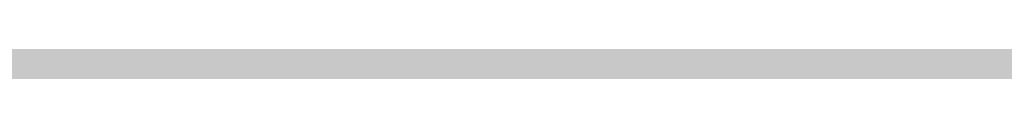
# Model space of a CAD drawing. Units: millimetres. Extents: x 0 to 2267, y 0 to 1823.
# Tile 198 of 256: x 1838.83 to 1841.442, y 1127.423 to 1127.462. Entities that reach past the tile are written whole.
import ezdxf

# ---------------------------------------------------------------- set-up
doc = ezdxf.new("R2010")
doc.units = ezdxf.units.MM
doc.header["$MEASUREMENT"] = 0
doc.layers.add('M-HATC', color=252, linetype='Continuous', lineweight=18)

msp = doc.modelspace()

# ---------------------------------------------------------------- hatches: boundary and pattern name
at = {"layer": 'M-HATC'}
h = msp.add_hatch(color=256, dxfattribs=at)
h.dxf.hatch_style = 1
h.paths.add_polyline_path([(2055.771, 1603.062), (1381.0868, 1603.062), (1381.0868, 1598.062), (2055.771, 1598.062)])
h.paths.add_polyline_path([(2055.771, 1598.062), (1381.0868, 1598.062), (1381.0868, 1593.062), (2055.771, 1593.062)])
h.paths.add_polyline_path([(2051.3074, 1536.7609), (1385.5504, 1536.7609), (1385.5504, 1526.7609), (1387.5504, 1526.7609), (1388.5366, 1525.0528), (1385.3319, 1521.2335), (1385.3319, 1521.2226), (2050.2542, 1522.7491), (2048.3212, 1525.0528), (2049.3074, 1526.7609), (2051.3074, 1526.7609)])
edge = h.paths.add_edge_path()
edge.add_arc((1847.5345, 1379.1492), 135, 222.603061, 222.890851, ccw=False)
edge.add_line((1748.1663, 1287.7656), (1683.0921, 1287.7656))
edge.add_arc((1583.7239, 1379.1492), 135, 317.109149, 317.396939, ccw=False)
edge.add_arc((1678.9686, 1290.6707), 5, 222.8909, 317.1091, ccw=False)
edge.add_arc((1774.2133, 1379.1492), 135, 222.603061, 222.890851, ccw=False)
edge.add_line((1674.8451, 1287.7656), (1609.7709, 1287.7656))
edge.add_arc((1510.4027, 1379.1492), 135, 317.109149, 317.396939, ccw=False)
edge.add_arc((1605.6474, 1290.6707), 5, 222.8909, 317.1091, ccw=False)
edge.add_arc((1700.8921, 1379.1492), 135, 222.603061, 222.890851, ccw=False)
edge.add_line((1601.5239, 1287.7656), (1536.4497, 1287.7656))
edge.add_arc((1437.0815, 1379.1492), 135, 317.109149, 317.396939, ccw=False)
edge.add_arc((1532.3262, 1290.6707), 5, 222.8909, 317.1091, ccw=False)
edge.add_arc((1627.5709, 1379.1492), 135, 222.603061, 222.890851, ccw=False)
edge.add_line((1528.2027, 1287.7656), (1505.9289, 1287.7656))
edge.add_spline(control_points=[(1505.9289, 1287.7656), (1504.2622, 1287.7656), (1504.2622, 1282.7656), (1505.9289, 1282.7656)], knot_values=[0, 0, 0, 0, 5, 5, 5, 5], degree=3, periodic=0)
edge.add_line((1505.9289, 1282.7656), (1930.9289, 1282.7656))
edge.add_spline(control_points=[(1930.9289, 1282.7656), (1932.5956, 1282.7656), (1932.5956, 1287.7656), (1930.9289, 1287.7656)], knot_values=[0, 0, 0, 0, 5, 5, 5, 5], degree=3, periodic=0)
edge.add_line((1930.9289, 1287.7656), (1903.0557, 1287.7656))
edge.add_arc((1803.6875, 1379.1492), 135, 317.109149, 317.396939, ccw=False)
edge.add_arc((1898.9322, 1290.6707), 5, 222.8909, 317.1091, ccw=False)
edge.add_arc((1994.1769, 1379.1492), 135, 222.603061, 222.890851, ccw=False)
edge.add_line((1894.8087, 1287.7656), (1829.7345, 1287.7656))
edge.add_arc((1730.3663, 1379.1492), 135, 317.109149, 317.396939, ccw=False)
edge.add_arc((1825.611, 1290.6707), 5, 222.8909, 317.1091, ccw=False)
edge.add_arc((1920.8557, 1379.1492), 135, 222.603061, 222.890851, ccw=False)
edge.add_line((1821.4875, 1287.7656), (1756.4133, 1287.7656))
edge.add_arc((1657.0451, 1379.1492), 135, 317.109149, 317.396939, ccw=False)
edge.add_arc((1752.2898, 1290.6707), 5, 222.8909, 317.1091, ccw=False)
edge = h.paths.add_edge_path()
edge.add_spline(control_points=[(1843.4289, 1227.2475), (1845.0956, 1227.2475), (1845.0956, 1232.2475), (1843.4289, 1232.2475)], knot_values=[0, 0, 0, 0, 5, 5, 5, 5], degree=3, periodic=0)
edge.add_line((1843.4289, 1232.2475), (1593.4289, 1232.2475))
edge.add_spline(control_points=[(1593.4289, 1232.2475), (1591.7622, 1232.2475), (1591.7622, 1227.2475), (1593.4289, 1227.2475)], knot_values=[0, 0, 0, 0, 5, 5, 5, 5], degree=3, periodic=0)
edge.add_line((1593.4289, 1227.2475), (1843.4289, 1227.2475))
h.paths.add_polyline_path([(1905.9289, 1127.4171), (1530.9289, 1127.4171, 0.414214), (1520.9289, 1117.4171), (1530.9289, 1117.4171), (1915.9289, 1117.4171, 0.414214)])
edge = h.paths.add_edge_path()
edge.add_arc((1397.0858, 1498.4078), 12.7299, 90.78215, 190.87871, ccw=False)
edge.add_line((1396.912, 1511.1365), (1428.0097, 1511.3488))
edge.add_line((1428.0097, 1511.3488), (1433.0097, 1511.3488))
edge.add_line((1433.0097, 1511.3488), (1434.439, 1511.3488))
edge.add_arc((1419.474, 1498.0804), 20, 41.561, 74.08211)
edge.add_line((1424.9592, 1517.3135), (1399.9351, 1517.2561))
edge.add_spline(control_points=[(1399.9307, 1517.2561), (1399.884, 1517.2131), (1399.8328, 1517.1689), (1399.7774, 1517.1236)], knot_values=[11.567499, 11.567499, 11.567499, 11.567499, 11.814249, 11.814249, 11.814249, 11.814249], degree=3, periodic=0)
edge.add_spline(control_points=[(1399.6328, 1517.0099), (1399.5831, 1516.9721), (1399.5307, 1516.9338), (1399.4759, 1516.8947)], knot_values=[11.167718, 11.167718, 11.167718, 11.167718, 11.365188, 11.365188, 11.365188, 11.365188], degree=3, periodic=0)
edge.add_spline(control_points=[(1399.3398, 1516.8001), (1399.1514, 1516.6719), (1398.9384, 1516.5377), (1398.704, 1516.3994)], knot_values=[10.376405, 10.376405, 10.376405, 10.376405, 11.00994, 11.00994, 11.00994, 11.00994], degree=3, periodic=0)
edge.add_spline(control_points=[(1398.6572, 1516.3719), (1398.5789, 1516.326), (1398.4983, 1516.2797), (1398.4155, 1516.2331)], knot_values=[10.125175, 10.125175, 10.125175, 10.125175, 10.334406, 10.334406, 10.334406, 10.334406], degree=3, periodic=0)
edge.add_spline(control_points=[(1398.2642, 1516.1487), (1398.196, 1516.1111), (1398.1263, 1516.0732), (1398.0555, 1516.0351)], knot_values=[9.832246, 9.832246, 9.832246, 9.832246, 9.999658, 9.999658, 9.999658, 9.999658], degree=3, periodic=0)
edge.add_spline(control_points=[(1397.9987, 1516.0048), (1397.7312, 1515.8621), (1397.446, 1515.7171), (1397.1466, 1515.5714)], knot_values=[9.161808, 9.161808, 9.161808, 9.161808, 9.787769, 9.787769, 9.787769, 9.787769], degree=3, periodic=0)
edge.add_spline(control_points=[(1397.1466, 1515.5714), (1396.8418, 1515.423), (1396.5222, 1515.274), (1396.1914, 1515.1262)], knot_values=[8.524455, 8.524455, 8.524455, 8.524455, 9.161808, 9.161808, 9.161808, 9.161808], degree=3, periodic=0)
edge.add_spline(control_points=[(1396.0777, 1515.0756), (1395.9854, 1515.0348), (1395.8922, 1514.994), (1395.7983, 1514.9534)], knot_values=[8.275193, 8.275193, 8.275193, 8.275193, 8.451726, 8.451726, 8.451726, 8.451726], degree=3, periodic=0)
edge.add_spline(control_points=[(1395.6018, 1514.8691), (1395.4997, 1514.8257), (1395.3968, 1514.7824), (1395.2932, 1514.7394)], knot_values=[7.962917, 7.962917, 7.962917, 7.962917, 8.152764, 8.152764, 8.152764, 8.152764], degree=3, periodic=0)
edge.add_spline(control_points=[(1395.2116, 1514.7057), (1394.8278, 1514.5475), (1394.4345, 1514.3929), (1394.0364, 1514.2442)], knot_values=[7.21254, 7.21254, 7.21254, 7.21254, 7.913148, 7.913148, 7.913148, 7.913148], degree=3, periodic=0)
edge.add_spline(control_points=[(1394.0364, 1514.2442), (1393.7076, 1514.1214), (1393.3754, 1514.0027), (1393.0427, 1513.8895)], knot_values=[6.633733, 6.633733, 6.633733, 6.633733, 7.21254, 7.21254, 7.21254, 7.21254], degree=3, periodic=0)
edge.add_spline(control_points=[(1392.8214, 1513.815), (1392.7198, 1513.7812), (1392.6181, 1513.7479), (1392.5166, 1513.7152)], knot_values=[6.328796, 6.328796, 6.328796, 6.328796, 6.505493, 6.505493, 6.505493, 6.505493], degree=3, periodic=0)
edge.add_spline(control_points=[(1392.5166, 1513.7152), (1392.3187, 1513.6515), (1392.1212, 1513.59), (1391.9244, 1513.531)], knot_values=[5.984605, 5.984605, 5.984605, 5.984605, 6.328796, 6.328796, 6.328796, 6.328796], degree=3, periodic=0)
edge.add_spline(control_points=[(1391.7915, 1513.4915), (1391.3122, 1513.3501), (1390.8384, 1513.2239), (1390.3784, 1513.1171)], knot_values=[5.066697, 5.066697, 5.066697, 5.066697, 5.907055, 5.907055, 5.907055, 5.907055], degree=3, periodic=0)
edge.add_spline(control_points=[(1390.3784, 1513.1171), (1390.1797, 1513.071), (1389.9836, 1513.0284), (1389.7907, 1512.9899)], knot_values=[4.70367, 4.70367, 4.70367, 4.70367, 5.066695, 5.066695, 5.066695, 5.066695], degree=3, periodic=0)
edge.add_spline(control_points=[(1389.422, 1512.9204), (1389.2459, 1512.8892), (1389.0729, 1512.8617), (1388.9036, 1512.8381)], knot_values=[4.130571, 4.130571, 4.130571, 4.130571, 4.469816, 4.469816, 4.469816, 4.469816], degree=3, periodic=0)
edge.add_spline(control_points=[(1388.9036, 1512.8381), (1388.591, 1512.7946), (1388.2911, 1512.7644), (1388.0071, 1512.7494)], knot_values=[3.504031, 3.504031, 3.504031, 3.504031, 4.130571, 4.130571, 4.130571, 4.130571], degree=3, periodic=0)
edge.add_spline(control_points=[(1387.9356, 1512.7459), (1387.8538, 1512.7423), (1387.7733, 1512.74), (1387.6944, 1512.739)], knot_values=[3.268866, 3.268866, 3.268866, 3.268866, 3.451164, 3.451164, 3.451164, 3.451164], degree=3, periodic=0)
edge.add_spline(control_points=[(1387.3351, 1512.7443), (1387.2076, 1512.7499), (1387.0847, 1512.7597), (1386.967, 1512.7739)], knot_values=[2.670686, 2.670686, 2.670686, 2.670686, 2.984, 2.984, 2.984, 2.984], degree=3, periodic=0)
edge.add_spline(control_points=[(1386.8327, 1512.7922), (1386.8209, 1512.7941), (1386.8092, 1512.7959), (1386.7975, 1512.7979)], knot_values=[2.516981, 2.516981, 2.516981, 2.516981, 2.549528, 2.549528, 2.549528, 2.549528], degree=3, periodic=0)
edge.add_spline(control_points=[(1386.4526, 1512.8735), (1386.4257, 1512.881), (1386.3993, 1512.889), (1386.3733, 1512.8972)], knot_values=[2.095869, 2.095869, 2.095869, 2.095869, 2.17941, 2.17941, 2.17941, 2.17941], degree=3, periodic=0)
edge.add_spline(control_points=[(1386.0691, 1513.0189), (1386.0634, 1513.0217), (1386.0577, 1513.0246), (1386.052, 1513.0275)], knot_values=[1.72453, 1.72453, 1.72453, 1.72453, 1.745933, 1.745933, 1.745933, 1.745933], degree=3, periodic=0)
edge.add_arc((1399.474, 1498.0804), 20, 131.82432, 180)
edge.add_arc((1630.3336, 1505.5484), 250.9708, 181.705176, 236.427975)
edge.add_arc((1605.3399, 1483.3044), 218.7822, 238.660829, 243.34961)
edge.add_arc((1647.0911, 1510.3592), 262.8986, 183.129836, 237.853442, ccw=False)
h.paths.add_polyline_path([(1406.5369, 1391.9644, 0.149382), (1491.5506, 1296.4418, -0.129517)], flags=17)
edge = h.paths.add_edge_path()
edge.add_arc((2037.3838, 1498.0804), 20, 0, 48.26587)
edge.add_spline(control_points=[(2050.6973, 1513.0052), (2050.6512, 1512.9847), (2050.6034, 1512.9655), (2050.5539, 1512.9477)], knot_values=[1.835652, 1.835652, 1.835652, 1.835652, 2.000781, 2.000781, 2.000781, 2.000781], degree=3, periodic=0)
edge.add_spline(control_points=[(2050.4616, 1512.9166), (2050.479, 1512.9221), (2050.4963, 1512.9277), (2050.5133, 1512.9335)], knot_values=[2.045477, 2.045477, 2.045477, 2.045477, 2.101389, 2.101389, 2.101389, 2.101389], degree=3, periodic=0)
edge.add_spline(control_points=[(2050.129, 1512.8342), (2050.1984, 1512.8473), (2050.2657, 1512.8623), (2050.3308, 1512.8792)], knot_values=[2.237629, 2.237629, 2.237629, 2.237629, 2.435841, 2.435841, 2.435841, 2.435841], degree=3, periodic=0)
edge.add_spline(control_points=[(2050.0946, 1512.8278), (2050.1061, 1512.8299), (2050.1176, 1512.832), (2050.129, 1512.8342)], knot_values=[2.435841, 2.435841, 2.435841, 2.435841, 2.468321, 2.468321, 2.468321, 2.468321], degree=3, periodic=0)
edge.add_spline(control_points=[(2049.7843, 1512.7851), (2049.8552, 1512.7922), (2049.9243, 1512.8008), (2049.9917, 1512.8109)], knot_values=[2.563852, 2.563852, 2.563852, 2.563852, 2.748541, 2.748541, 2.748541, 2.748541], degree=3, periodic=0)
edge.add_spline(control_points=[(2049.4052, 1512.7617), (2049.5364, 1512.7653), (2049.6629, 1512.773), (2049.7843, 1512.7851)], knot_values=[2.748541, 2.748541, 2.748541, 2.748541, 3.064882, 3.064882, 3.064882, 3.064882], degree=3, periodic=0)
edge.add_spline(control_points=[(2049.1698, 1512.7597), (2049.2336, 1512.7591), (2049.2965, 1512.7594), (2049.3584, 1512.7606)], knot_values=[3.102309, 3.102309, 3.102309, 3.102309, 3.2503, 3.2503, 3.2503, 3.2503], degree=3, periodic=0)
edge.add_spline(control_points=[(2048.8573, 1512.7691), (2048.9638, 1512.7638), (2049.068, 1512.7606), (2049.1698, 1512.7597)], knot_values=[3.2503, 3.2503, 3.2503, 3.2503, 3.486069, 3.486069, 3.486069, 3.486069], degree=3, periodic=0)
edge.add_spline(control_points=[(2048.6924, 1512.7789), (2048.3729, 1512.8009), (2048.0345, 1512.8411), (2047.6817, 1512.897)], knot_values=[3.606429, 3.606429, 3.606429, 3.606429, 4.2989, 4.2989, 4.2989, 4.2989], degree=3, periodic=0)
edge.add_spline(control_points=[(2047.6817, 1512.897), (2047.5458, 1512.9185), (2047.4077, 1512.9424), (2047.2678, 1512.9685)], knot_values=[4.2989, 4.2989, 4.2989, 4.2989, 4.565769, 4.565769, 4.565769, 4.565769], degree=3, periodic=0)
edge.add_spline(control_points=[(2047.2678, 1512.9685), (2047.1449, 1512.9914), (2047.0207, 1513.016), (2046.8951, 1513.0422)], knot_values=[4.565769, 4.565769, 4.565769, 4.565769, 4.799971, 4.799971, 4.799971, 4.799971], degree=3, periodic=0)
edge.add_spline(control_points=[(2046.8951, 1513.0422), (2046.5286, 1513.1188), (2046.1513, 1513.209), (2045.7676, 1513.3107)], knot_values=[4.799971, 4.799971, 4.799971, 4.799971, 5.483718, 5.483718, 5.483718, 5.483718], degree=3, periodic=0)
edge.add_spline(control_points=[(2045.7676, 1513.3107), (2045.3724, 1513.4154), (2044.9704, 1513.5322), (2044.5662, 1513.6588)], knot_values=[5.483718, 5.483718, 5.483718, 5.483718, 6.187866, 6.187866, 6.187866, 6.187866], degree=3, periodic=0)
edge.add_spline(control_points=[(2044.5662, 1513.6588), (2044.4149, 1513.7061), (2044.2633, 1513.7549), (2044.1116, 1513.8048)], knot_values=[6.187866, 6.187866, 6.187866, 6.187866, 6.451551, 6.451551, 6.451551, 6.451551], degree=3, periodic=0)
edge.add_spline(control_points=[(2044.1116, 1513.8048), (2043.9967, 1513.8427), (2043.8817, 1513.8813), (2043.7668, 1513.9205)], knot_values=[6.451551, 6.451551, 6.451551, 6.451551, 6.651434, 6.651434, 6.651434, 6.651434], degree=3, periodic=0)
edge.add_spline(control_points=[(2043.7668, 1513.9205), (2043.3716, 1514.0554), (2042.9774, 1514.1979), (2042.5886, 1514.3458)], knot_values=[6.651434, 6.651434, 6.651434, 6.651434, 7.338879, 7.338879, 7.338879, 7.338879], degree=3, periodic=0)
edge.add_spline(control_points=[(2042.5886, 1514.3458), (2042.1643, 1514.5071), (2041.7465, 1514.6749), (2041.3409, 1514.846)], knot_values=[7.338879, 7.338879, 7.338879, 7.338879, 8.089209, 8.089209, 8.089209, 8.089209], degree=3, periodic=0)
edge.add_spline(control_points=[(2041.3409, 1514.846), (2041.1028, 1514.9465), (2040.869, 1515.0481), (2040.6405, 1515.1502)], knot_values=[8.089209, 8.089209, 8.089209, 8.089209, 8.529587, 8.529587, 8.529587, 8.529587], degree=3, periodic=0)
edge.add_spline(control_points=[(2040.51, 1515.2089), (2040.0824, 1515.4022), (2039.6747, 1515.5971), (2039.295, 1515.7894)], knot_values=[8.613818, 8.613818, 8.613818, 8.613818, 9.44571, 9.44571, 9.44571, 9.44571], degree=3, periodic=0)
edge.add_spline(control_points=[(2039.295, 1515.7894), (2039.0618, 1515.9075), (2038.8391, 1516.0246), (2038.6288, 1516.1398)], knot_values=[9.44571, 9.44571, 9.44571, 9.44571, 9.956404, 9.956404, 9.956404, 9.956404], degree=3, periodic=0)
edge.add_spline(control_points=[(2038.6288, 1516.1398), (2038.5187, 1516.2001), (2038.4121, 1516.2598), (2038.309, 1516.3189)], knot_values=[9.956404, 9.956404, 9.956404, 9.956404, 10.223542, 10.223542, 10.223542, 10.223542], degree=3, periodic=0)
edge.add_spline(control_points=[(2038.309, 1516.3189), (2038.2138, 1516.3735), (2038.1216, 1516.4276), (2038.0328, 1516.481)], knot_values=[10.223542, 10.223542, 10.223542, 10.223542, 10.47051, 10.47051, 10.47051, 10.47051], degree=3, periodic=0)
edge.add_spline(control_points=[(2038.0328, 1516.481), (2037.7855, 1516.6296), (2037.5639, 1516.773), (2037.3722, 1516.909)], knot_values=[10.47051, 10.47051, 10.47051, 10.47051, 11.15767, 11.15767, 11.15767, 11.15767], degree=3, periodic=0)
edge.add_spline(control_points=[(2037.3722, 1516.909), (2037.2789, 1516.9752), (2037.1927, 1517.0396), (2037.1142, 1517.102)], knot_values=[11.15767, 11.15767, 11.15767, 11.15767, 11.49227, 11.49227, 11.49227, 11.49227], degree=3, periodic=0)
edge.add_spline(control_points=[(2036.8564, 1517.3259), (2036.9148, 1517.2692), (2036.9814, 1517.2103), (2037.0557, 1517.1492)], knot_values=[11.577341, 11.577341, 11.577341, 11.577341, 11.91035, 11.91035, 11.91035, 11.91035], degree=3, periodic=0)
edge.add_spline(control_points=[(2036.8074, 1517.3748), (2036.823, 1517.3587), (2036.8393, 1517.3424), (2036.8564, 1517.3259)], knot_values=[11.91035, 11.91035, 11.91035, 11.91035, 12.007402, 12.007402, 12.007402, 12.007402], degree=3, periodic=0)
edge.add_spline(control_points=[(2036.7017, 1517.494), (2036.7104, 1517.483), (2036.7196, 1517.4719), (2036.7291, 1517.4606)], knot_values=[12.184155, 12.184155, 12.184155, 12.184155, 12.255409, 12.255409, 12.255409, 12.255409], degree=3, periodic=0)
edge.add_spline(control_points=[(2036.6159, 1517.6205), (2036.62, 1517.613), (2036.6243, 1517.6055), (2036.6289, 1517.5979)], knot_values=[12.487913, 12.487913, 12.487913, 12.487913, 12.541035, 12.541035, 12.541035, 12.541035], degree=3, periodic=0)
edge.add_spline(control_points=[(2036.5635, 1517.786), (2036.5637, 1517.7794), (2036.5642, 1517.7726), (2036.565, 1517.7658)], knot_values=[12.911761, 12.911761, 12.911761, 12.911761, 12.968286, 12.968286, 12.968286, 12.968286], degree=3, periodic=0)
edge.add_spline(control_points=[(2036.6166, 1517.9304), (2036.6125, 1517.9259), (2036.6086, 1517.9212), (2036.6049, 1517.9165)], knot_values=[13.382527, 13.382527, 13.382527, 13.382527, 13.433791, 13.433791, 13.433791, 13.433791], degree=3, periodic=0)
edge.add_spline(control_points=[(2036.749, 1518.017), (2036.7361, 1518.0116), (2036.7239, 1518.006), (2036.7124, 1518.0002)], knot_values=[13.726299, 13.726299, 13.726299, 13.726299, 13.809928, 13.809928, 13.809928, 13.809928], degree=3, periodic=0)
edge.add_spline(control_points=[(2036.8604, 1518.0528), (2036.8386, 1518.0474), (2036.8181, 1518.0416), (2036.7988, 1518.0353)], knot_values=[13.910887, 13.910887, 13.910887, 13.910887, 14.02153, 14.02153, 14.02153, 14.02153], degree=3, periodic=0)
edge.add_line((2036.9639, 1518.0804), (2032.3838, 1518.0804))
edge.add_line((2032.3838, 1518.0804), (2027.3838, 1518.0804))
edge.add_line((2027.3838, 1518.0804), (2022.3838, 1518.0804))
edge.add_line((2022.3838, 1518.0804), (2017.3838, 1518.0804))
edge.add_arc((2017.3838, 1498.0804), 20, 90, 138.439)
edge.add_line((2002.4188, 1511.3488), (2003.8481, 1511.3488))
edge.add_line((2003.8481, 1511.3488), (2008.8481, 1511.3488))
edge.add_line((2008.8481, 1511.3488), (2039.772, 1511.1377))
edge.add_arc((2039.772, 1498.4078), 12.7299, -10.87871, 90, ccw=False)
edge.add_arc((1789.7668, 1510.3592), 262.8986, 302.146558, 356.870164, ccw=False)
edge.add_arc((1831.5179, 1483.3044), 218.7822, 296.65039, 301.339171)
edge.add_arc((1806.5242, 1505.5484), 250.9708, 303.572025, 358.294824)
h.paths.add_polyline_path([(2030.321, 1391.9644, -0.129517), (1945.3072, 1296.4418, 0.149382)], flags=17)
edge = h.paths.add_edge_path()
edge.add_spline(control_points=[(2037.2464, 1518.0821), (2037.2898, 1518.081), (2037.3355, 1518.0804), (2037.3838, 1518.0804)], knot_values=[0.000012, 0.000012, 0.000012, 0.000012, 0.144754, 0.144754, 0.144754, 0.144754], degree=3, periodic=0)
edge.add_line((2037.3357, 1518.0804), (2037.0096, 1518.0804))
edge.add_spline(control_points=[(2037.0096, 1518.0804), (2036.9822, 1518.0768), (2036.956, 1518.0727), (2036.9312, 1518.0681)], knot_values=[14.13465, 14.13465, 14.13465, 14.13465, 14.247197, 14.247197, 14.247197, 14.247197], degree=3, periodic=0)
edge.add_spline(control_points=[(2036.9312, 1518.0681), (2036.9276, 1518.0674), (2036.9241, 1518.0667), (2036.9205, 1518.0661)], knot_values=[14.118315, 14.118315, 14.118315, 14.118315, 14.13465, 14.13465, 14.13465, 14.13465], degree=3, periodic=0)
edge.add_spline(control_points=[(2036.9205, 1518.0661), (2036.9118, 1518.0644), (2036.9032, 1518.0626), (2036.8948, 1518.0608)], knot_values=[14.078086, 14.078086, 14.078086, 14.078086, 14.118315, 14.118315, 14.118315, 14.118315], degree=3, periodic=0)
edge.add_spline(control_points=[(2036.8948, 1518.0608), (2036.883, 1518.0583), (2036.8716, 1518.0556), (2036.8604, 1518.0528)], knot_values=[14.02153, 14.02153, 14.02153, 14.02153, 14.078086, 14.078086, 14.078086, 14.078086], degree=3, periodic=0)
edge.add_spline(control_points=[(2036.8604, 1518.0528), (2036.8386, 1518.0474), (2036.8181, 1518.0416), (2036.7988, 1518.0353)], knot_values=[13.910887, 13.910887, 13.910887, 13.910887, 14.02153, 14.02153, 14.02153, 14.02153], degree=3, periodic=0)
edge.add_spline(control_points=[(2036.7988, 1518.0353), (2036.7981, 1518.035), (2036.7974, 1518.0348), (2036.7967, 1518.0346)], knot_values=[13.906906, 13.906906, 13.906906, 13.906906, 13.910887, 13.910887, 13.910887, 13.910887], degree=3, periodic=0)
edge.add_spline(control_points=[(2036.7967, 1518.0346), (2036.7882, 1518.0318), (2036.7799, 1518.0289), (2036.7719, 1518.0259)], knot_values=[13.857826, 13.857826, 13.857826, 13.857826, 13.906906, 13.906906, 13.906906, 13.906906], degree=3, periodic=0)
edge.add_spline(control_points=[(2036.7719, 1518.0259), (2036.764, 1518.023), (2036.7564, 1518.02), (2036.749, 1518.017)], knot_values=[13.809928, 13.809928, 13.809928, 13.809928, 13.857826, 13.857826, 13.857826, 13.857826], degree=3, periodic=0)
edge.add_spline(control_points=[(2036.749, 1518.017), (2036.7361, 1518.0116), (2036.7239, 1518.006), (2036.7124, 1518.0002)], knot_values=[13.726299, 13.726299, 13.726299, 13.726299, 13.809928, 13.809928, 13.809928, 13.809928], degree=3, periodic=0)
edge.add_spline(control_points=[(2036.7124, 1518.0002), (2036.7121, 1518), (2036.7118, 1517.9999), (2036.7115, 1517.9997)], knot_values=[13.723993, 13.723993, 13.723993, 13.723993, 13.726299, 13.726299, 13.726299, 13.726299], degree=3, periodic=0)
edge.add_spline(control_points=[(2036.7115, 1517.9997), (2036.7063, 1517.9971), (2036.7013, 1517.9944), (2036.6965, 1517.9917)], knot_values=[13.686536, 13.686536, 13.686536, 13.686536, 13.723993, 13.723993, 13.723993, 13.723993], degree=3, periodic=0)
edge.add_spline(control_points=[(2036.6965, 1517.9917), (2036.6919, 1517.9891), (2036.6874, 1517.9865), (2036.6831, 1517.9839)], knot_values=[13.651251, 13.651251, 13.651251, 13.651251, 13.686536, 13.686536, 13.686536, 13.686536], degree=3, periodic=0)
edge.add_spline(control_points=[(2036.6831, 1517.9839), (2036.6764, 1517.9798), (2036.67, 1517.9757), (2036.6639, 1517.9714)], knot_values=[13.596804, 13.596804, 13.596804, 13.596804, 13.651251, 13.651251, 13.651251, 13.651251], degree=3, periodic=0)
edge.add_spline(control_points=[(2036.6639, 1517.9714), (2036.6636, 1517.9712), (2036.6633, 1517.9709), (2036.6629, 1517.9707)], knot_values=[13.593956, 13.593956, 13.593956, 13.593956, 13.596804, 13.596804, 13.596804, 13.596804], degree=3, periodic=0)
edge.add_spline(control_points=[(2036.6629, 1517.9707), (2036.6603, 1517.9689), (2036.6577, 1517.967), (2036.6552, 1517.9651)], knot_values=[13.570322, 13.570322, 13.570322, 13.570322, 13.593956, 13.593956, 13.593956, 13.593956], degree=3, periodic=0)
edge.add_spline(control_points=[(2036.6552, 1517.9651), (2036.6525, 1517.9631), (2036.6499, 1517.9611), (2036.6474, 1517.9591)], knot_values=[13.545477, 13.545477, 13.545477, 13.545477, 13.570322, 13.570322, 13.570322, 13.570322], degree=3, periodic=0)
edge.add_spline(control_points=[(2036.6474, 1517.9591), (2036.6472, 1517.9589), (2036.6471, 1517.9588), (2036.6469, 1517.9587)], knot_values=[13.543931, 13.543931, 13.543931, 13.543931, 13.545477, 13.545477, 13.545477, 13.545477], degree=3, periodic=0)
edge.add_spline(control_points=[(2036.6469, 1517.9587), (2036.6412, 1517.9541), (2036.6358, 1517.9494), (2036.6307, 1517.9447)], knot_values=[13.488237, 13.488237, 13.488237, 13.488237, 13.543931, 13.543931, 13.543931, 13.543931], degree=3, periodic=0)
edge.add_spline(control_points=[(2036.6307, 1517.9447), (2036.6282, 1517.9423), (2036.6257, 1517.9399), (2036.6233, 1517.9374)], knot_values=[13.460307, 13.460307, 13.460307, 13.460307, 13.488237, 13.488237, 13.488237, 13.488237], degree=3, periodic=0)
edge.add_spline(control_points=[(2036.6233, 1517.9374), (2036.6215, 1517.9356), (2036.6198, 1517.9338), (2036.6181, 1517.932)], knot_values=[13.439712, 13.439712, 13.439712, 13.439712, 13.460307, 13.460307, 13.460307, 13.460307], degree=3, periodic=0)
edge.add_spline(control_points=[(2036.6181, 1517.932), (2036.6176, 1517.9315), (2036.6171, 1517.9309), (2036.6166, 1517.9304)], knot_values=[13.433791, 13.433791, 13.433791, 13.433791, 13.439712, 13.439712, 13.439712, 13.439712], degree=3, periodic=0)
edge.add_spline(control_points=[(2036.6166, 1517.9304), (2036.6125, 1517.9259), (2036.6086, 1517.9212), (2036.6049, 1517.9165)], knot_values=[13.382527, 13.382527, 13.382527, 13.382527, 13.433791, 13.433791, 13.433791, 13.433791], degree=3, periodic=0)
edge.add_spline(control_points=[(2036.6049, 1517.9165), (2036.6026, 1517.9135), (2036.6004, 1517.9104), (2036.5982, 1517.9074)], knot_values=[13.350017, 13.350017, 13.350017, 13.350017, 13.382527, 13.382527, 13.382527, 13.382527], degree=3, periodic=0)
edge.add_spline(control_points=[(2036.5982, 1517.9074), (2036.5972, 1517.9059), (2036.5962, 1517.9043), (2036.5952, 1517.9028)], knot_values=[13.333922, 13.333922, 13.333922, 13.333922, 13.350017, 13.350017, 13.350017, 13.350017], degree=3, periodic=0)
edge.add_spline(control_points=[(2036.5952, 1517.9028), (2036.5945, 1517.9018), (2036.5939, 1517.9009), (2036.5933, 1517.8999)], knot_values=[13.323828, 13.323828, 13.323828, 13.323828, 13.333922, 13.333922, 13.333922, 13.333922], degree=3, periodic=0)
edge.add_spline(control_points=[(2036.5933, 1517.8999), (2036.5905, 1517.8955), (2036.5879, 1517.8909), (2036.5855, 1517.8864)], knot_values=[13.277545, 13.277545, 13.277545, 13.277545, 13.323828, 13.323828, 13.323828, 13.323828], degree=3, periodic=0)
edge.add_spline(control_points=[(2036.5855, 1517.8864), (2036.5836, 1517.8827), (2036.5817, 1517.8789), (2036.5801, 1517.8751)], knot_values=[13.240119, 13.240119, 13.240119, 13.240119, 13.277545, 13.277545, 13.277545, 13.277545], degree=3, periodic=0)
edge.add_spline(control_points=[(2036.5801, 1517.8751), (2036.5795, 1517.8739), (2036.579, 1517.8727), (2036.5785, 1517.8715)], knot_values=[13.228211, 13.228211, 13.228211, 13.228211, 13.240119, 13.240119, 13.240119, 13.240119], degree=3, periodic=0)
edge.add_spline(control_points=[(2036.5785, 1517.8715), (2036.578, 1517.8702), (2036.5774, 1517.869), (2036.5769, 1517.8677)], knot_values=[13.215717, 13.215717, 13.215717, 13.215717, 13.228211, 13.228211, 13.228211, 13.228211], degree=3, periodic=0)
edge.add_spline(control_points=[(2036.5769, 1517.8677), (2036.5755, 1517.864), (2036.5741, 1517.8603), (2036.5729, 1517.8565)], knot_values=[13.179847, 13.179847, 13.179847, 13.179847, 13.215717, 13.215717, 13.215717, 13.215717], degree=3, periodic=0)
edge.add_spline(control_points=[(2036.5729, 1517.8565), (2036.5713, 1517.8515), (2036.5699, 1517.8464), (2036.5687, 1517.8413)], knot_values=[13.132017, 13.132017, 13.132017, 13.132017, 13.179847, 13.179847, 13.179847, 13.179847], degree=3, periodic=0)
edge.add_spline(control_points=[(2036.5687, 1517.8413), (2036.5684, 1517.8402), (2036.5682, 1517.8392), (2036.568, 1517.8382)], knot_values=[13.122482, 13.122482, 13.122482, 13.122482, 13.132017, 13.132017, 13.132017, 13.132017], degree=3, periodic=0)
edge.add_spline(control_points=[(2036.568, 1517.8382), (2036.5676, 1517.8363), (2036.5672, 1517.8345), (2036.5669, 1517.8327)], knot_values=[13.105592, 13.105592, 13.105592, 13.105592, 13.122482, 13.122482, 13.122482, 13.122482], degree=3, periodic=0)
edge.add_spline(control_points=[(2036.5669, 1517.8327), (2036.5662, 1517.8292), (2036.5657, 1517.8257), (2036.5652, 1517.8222)], knot_values=[13.074063, 13.074063, 13.074063, 13.074063, 13.105592, 13.105592, 13.105592, 13.105592], degree=3, periodic=0)
edge.add_spline(control_points=[(2036.5652, 1517.8222), (2036.5652, 1517.8222), (2036.5652, 1517.8222), (2036.5652, 1517.8222)], knot_values=[13.074043, 13.074043, 13.074043, 13.074043, 13.074063, 13.074063, 13.074063, 13.074063], degree=3, periodic=0)
edge.add_spline(control_points=[(2036.5652, 1517.8222), (2036.5644, 1517.8164), (2036.5639, 1517.8106), (2036.5636, 1517.8046)], knot_values=[13.021884, 13.021884, 13.021884, 13.021884, 13.074043, 13.074043, 13.074043, 13.074043], degree=3, periodic=0)
edge.add_spline(control_points=[(2036.5636, 1517.8046), (2036.5636, 1517.804), (2036.5636, 1517.8034), (2036.5635, 1517.8028)], knot_values=[13.01674, 13.01674, 13.01674, 13.01674, 13.021884, 13.021884, 13.021884, 13.021884], degree=3, periodic=0)
edge.add_spline(control_points=[(2036.5635, 1517.8028), (2036.5634, 1517.8005), (2036.5634, 1517.7982), (2036.5634, 1517.7958)], knot_values=[12.996438, 12.996438, 12.996438, 12.996438, 13.01674, 13.01674, 13.01674, 13.01674], degree=3, periodic=0)
edge.add_spline(control_points=[(2036.5634, 1517.7958), (2036.5633, 1517.7926), (2036.5634, 1517.7893), (2036.5635, 1517.786)], knot_values=[12.968286, 12.968286, 12.968286, 12.968286, 12.996438, 12.996438, 12.996438, 12.996438], degree=3, periodic=0)
edge.add_spline(control_points=[(2036.5635, 1517.786), (2036.5637, 1517.7794), (2036.5642, 1517.7726), (2036.565, 1517.7658)], knot_values=[12.911761, 12.911761, 12.911761, 12.911761, 12.968286, 12.968286, 12.968286, 12.968286], degree=3, periodic=0)
edge.add_spline(control_points=[(2036.565, 1517.7658), (2036.565, 1517.7657), (2036.565, 1517.7656), (2036.565, 1517.7656)], knot_values=[12.911017, 12.911017, 12.911017, 12.911017, 12.911761, 12.911761, 12.911761, 12.911761], degree=3, periodic=0)
edge.add_spline(control_points=[(2036.565, 1517.7656), (2036.5654, 1517.7625), (2036.5658, 1517.7593), (2036.5663, 1517.7562)], knot_values=[12.88528, 12.88528, 12.88528, 12.88528, 12.911017, 12.911017, 12.911017, 12.911017], degree=3, periodic=0)
edge.add_spline(control_points=[(2036.5663, 1517.7562), (2036.5667, 1517.7534), (2036.5672, 1517.7506), (2036.5677, 1517.7478)], knot_values=[12.862519, 12.862519, 12.862519, 12.862519, 12.88528, 12.88528, 12.88528, 12.88528], degree=3, periodic=0)
edge.add_spline(control_points=[(2036.5677, 1517.7478), (2036.5678, 1517.7474), (2036.5679, 1517.7469), (2036.568, 1517.7465)], knot_values=[12.858885, 12.858885, 12.858885, 12.858885, 12.862519, 12.862519, 12.862519, 12.862519], degree=3, periodic=0)
edge.add_spline(control_points=[(2036.568, 1517.7465), (2036.5692, 1517.7399), (2036.5707, 1517.7332), (2036.5724, 1517.7264)], knot_values=[12.8053, 12.8053, 12.8053, 12.8053, 12.858885, 12.858885, 12.858885, 12.858885], degree=3, periodic=0)
edge.add_spline(control_points=[(2036.5724, 1517.7264), (2036.5734, 1517.7226), (2036.5745, 1517.7187), (2036.5756, 1517.7149)], knot_values=[12.775176, 12.775176, 12.775176, 12.775176, 12.8053, 12.8053, 12.8053, 12.8053], degree=3, periodic=0)
edge.add_spline(control_points=[(2036.5756, 1517.7149), (2036.5763, 1517.7125), (2036.577, 1517.7102), (2036.5778, 1517.7078)], knot_values=[12.756759, 12.756759, 12.756759, 12.756759, 12.775176, 12.775176, 12.775176, 12.775176], degree=3, periodic=0)
edge.add_spline(control_points=[(2036.5778, 1517.7078), (2036.5781, 1517.7067), (2036.5784, 1517.7057), (2036.5787, 1517.7047)], knot_values=[12.748742, 12.748742, 12.748742, 12.748742, 12.756759, 12.756759, 12.756759, 12.756759], degree=3, periodic=0)
edge.add_spline(control_points=[(2036.5787, 1517.7047), (2036.5808, 1517.6983), (2036.5831, 1517.6919), (2036.5856, 1517.6854)], knot_values=[12.69959, 12.69959, 12.69959, 12.69959, 12.748742, 12.748742, 12.748742, 12.748742], degree=3, periodic=0)
edge.add_spline(control_points=[(2036.5856, 1517.6854), (2036.5876, 1517.68), (2036.5898, 1517.6746), (2036.5921, 1517.6692)], knot_values=[12.659038, 12.659038, 12.659038, 12.659038, 12.69959, 12.69959, 12.69959, 12.69959], degree=3, periodic=0)
edge.add_spline(control_points=[(2036.5921, 1517.6692), (2036.594, 1517.6648), (2036.5959, 1517.6605), (2036.5979, 1517.6561)], knot_values=[12.626806, 12.626806, 12.626806, 12.626806, 12.659038, 12.659038, 12.659038, 12.659038], degree=3, periodic=0)
edge.add_spline(control_points=[(2036.5979, 1517.6561), (2036.5984, 1517.6551), (2036.5989, 1517.6541), (2036.5993, 1517.6531)], knot_values=[12.619394, 12.619394, 12.619394, 12.619394, 12.626806, 12.626806, 12.626806, 12.626806], degree=3, periodic=0)
edge.add_spline(control_points=[(2036.5993, 1517.6531), (2036.6043, 1517.6424), (2036.6099, 1517.6315), (2036.6159, 1517.6205)], knot_values=[12.541039, 12.541039, 12.541039, 12.541039, 12.619394, 12.619394, 12.619394, 12.619394], degree=3, periodic=0)
edge.add_spline(control_points=[(2036.6159, 1517.6205), (2036.6159, 1517.6205), (2036.6159, 1517.6205), (2036.6159, 1517.6205)], knot_values=[12.541035, 12.541035, 12.541035, 12.541035, 12.541039, 12.541039, 12.541039, 12.541039], degree=3, periodic=0)
edge.add_spline(control_points=[(2036.6159, 1517.6205), (2036.62, 1517.613), (2036.6243, 1517.6055), (2036.6289, 1517.5979)], knot_values=[12.487913, 12.487913, 12.487913, 12.487913, 12.541035, 12.541035, 12.541035, 12.541035], degree=3, periodic=0)
edge.add_spline(control_points=[(2036.6289, 1517.5979), (2036.6326, 1517.5916), (2036.6365, 1517.5853), (2036.6406, 1517.5789)], knot_values=[12.443982, 12.443982, 12.443982, 12.443982, 12.487913, 12.487913, 12.487913, 12.487913], degree=3, periodic=0)
edge.add_spline(control_points=[(2036.6406, 1517.5789), (2036.6414, 1517.5776), (2036.6423, 1517.5763), (2036.6431, 1517.5749)], knot_values=[12.434996, 12.434996, 12.434996, 12.434996, 12.443982, 12.443982, 12.443982, 12.443982], degree=3, periodic=0)
edge.add_spline(control_points=[(2036.6431, 1517.5749), (2036.6531, 1517.5596), (2036.6639, 1517.5439), (2036.6756, 1517.528)], knot_values=[12.329647, 12.329647, 12.329647, 12.329647, 12.434996, 12.434996, 12.434996, 12.434996], degree=3, periodic=0)
edge.add_spline(control_points=[(2036.6756, 1517.528), (2036.6839, 1517.5168), (2036.6925, 1517.5055), (2036.7017, 1517.494)], knot_values=[12.255409, 12.255409, 12.255409, 12.255409, 12.329647, 12.329647, 12.329647, 12.329647], degree=3, periodic=0)
edge.add_spline(control_points=[(2036.7017, 1517.494), (2036.7104, 1517.483), (2036.7196, 1517.4719), (2036.7291, 1517.4606)], knot_values=[12.184155, 12.184155, 12.184155, 12.184155, 12.255409, 12.255409, 12.255409, 12.255409], degree=3, periodic=0)
edge.add_spline(control_points=[(2036.7291, 1517.4606), (2036.7436, 1517.4435), (2036.759, 1517.4262), (2036.7753, 1517.4085)], knot_values=[12.075961, 12.075961, 12.075961, 12.075961, 12.184155, 12.184155, 12.184155, 12.184155], degree=3, periodic=0)
edge.add_spline(control_points=[(2036.7753, 1517.4085), (2036.7763, 1517.4075), (2036.7773, 1517.4064), (2036.7783, 1517.4054)], knot_values=[12.069502, 12.069502, 12.069502, 12.069502, 12.075961, 12.075961, 12.075961, 12.075961], degree=3, periodic=0)
edge.add_spline(control_points=[(2036.7783, 1517.4054), (2036.7877, 1517.3953), (2036.7974, 1517.385), (2036.8074, 1517.3748)], knot_values=[12.007402, 12.007402, 12.007402, 12.007402, 12.069502, 12.069502, 12.069502, 12.069502], degree=3, periodic=0)
edge.add_spline(control_points=[(2036.8074, 1517.3748), (2036.823, 1517.3587), (2036.8393, 1517.3424), (2036.8564, 1517.3259)], knot_values=[11.91035, 11.91035, 11.91035, 11.91035, 12.007402, 12.007402, 12.007402, 12.007402], degree=3, periodic=0)
edge.add_spline(control_points=[(2036.8564, 1517.3259), (2036.9148, 1517.2692), (2036.9814, 1517.2103), (2037.0557, 1517.1492)], knot_values=[11.577341, 11.577341, 11.577341, 11.577341, 11.91035, 11.91035, 11.91035, 11.91035], degree=3, periodic=0)
edge.add_spline(control_points=[(2037.0557, 1517.1492), (2037.0747, 1517.1336), (2037.0942, 1517.1179), (2037.1142, 1517.102)], knot_values=[11.49227, 11.49227, 11.49227, 11.49227, 11.577341, 11.577341, 11.577341, 11.577341], degree=3, periodic=0)
edge.add_spline(control_points=[(2037.1142, 1517.102), (2037.1927, 1517.0396), (2037.2789, 1516.9752), (2037.3722, 1516.909)], knot_values=[11.15767, 11.15767, 11.15767, 11.15767, 11.49227, 11.49227, 11.49227, 11.49227], degree=3, periodic=0)
edge.add_spline(control_points=[(2037.3722, 1516.909), (2037.5639, 1516.773), (2037.7855, 1516.6296), (2038.0328, 1516.481)], knot_values=[10.47051, 10.47051, 10.47051, 10.47051, 11.15767, 11.15767, 11.15767, 11.15767], degree=3, periodic=0)
edge.add_spline(control_points=[(2038.0328, 1516.481), (2038.1216, 1516.4276), (2038.2138, 1516.3735), (2038.309, 1516.3189)], knot_values=[10.223542, 10.223542, 10.223542, 10.223542, 10.47051, 10.47051, 10.47051, 10.47051], degree=3, periodic=0)
edge.add_spline(control_points=[(2038.309, 1516.3189), (2038.4121, 1516.2598), (2038.5187, 1516.2001), (2038.6288, 1516.1398)], knot_values=[9.956404, 9.956404, 9.956404, 9.956404, 10.223542, 10.223542, 10.223542, 10.223542], degree=3, periodic=0)
edge.add_spline(control_points=[(2038.6288, 1516.1398), (2038.8391, 1516.0246), (2039.0618, 1515.9075), (2039.295, 1515.7894)], knot_values=[9.44571, 9.44571, 9.44571, 9.44571, 9.956404, 9.956404, 9.956404, 9.956404], degree=3, periodic=0)
edge.add_spline(control_points=[(2039.295, 1515.7894), (2039.6747, 1515.5971), (2040.0824, 1515.4022), (2040.51, 1515.2089)], knot_values=[8.613818, 8.613818, 8.613818, 8.613818, 9.44571, 9.44571, 9.44571, 9.44571], degree=3, periodic=0)
edge.add_spline(control_points=[(2040.51, 1515.2089), (2040.5533, 1515.1893), (2040.5968, 1515.1697), (2040.6405, 1515.1502)], knot_values=[8.529587, 8.529587, 8.529587, 8.529587, 8.613818, 8.613818, 8.613818, 8.613818], degree=3, periodic=0)
edge.add_spline(control_points=[(2040.6405, 1515.1502), (2040.869, 1515.0481), (2041.1028, 1514.9465), (2041.3409, 1514.846)], knot_values=[8.089209, 8.089209, 8.089209, 8.089209, 8.529587, 8.529587, 8.529587, 8.529587], degree=3, periodic=0)
edge.add_spline(control_points=[(2041.3409, 1514.846), (2041.7465, 1514.6749), (2042.1643, 1514.5071), (2042.5886, 1514.3458)], knot_values=[7.338879, 7.338879, 7.338879, 7.338879, 8.089209, 8.089209, 8.089209, 8.089209], degree=3, periodic=0)
edge.add_spline(control_points=[(2042.5886, 1514.3458), (2042.9774, 1514.1979), (2043.3716, 1514.0554), (2043.7668, 1513.9205)], knot_values=[6.651434, 6.651434, 6.651434, 6.651434, 7.338879, 7.338879, 7.338879, 7.338879], degree=3, periodic=0)
edge.add_spline(control_points=[(2043.7668, 1513.9205), (2043.8817, 1513.8813), (2043.9967, 1513.8427), (2044.1116, 1513.8048)], knot_values=[6.451551, 6.451551, 6.451551, 6.451551, 6.651434, 6.651434, 6.651434, 6.651434], degree=3, periodic=0)
edge.add_spline(control_points=[(2044.1116, 1513.8048), (2044.2633, 1513.7549), (2044.4149, 1513.7061), (2044.5662, 1513.6588)], knot_values=[6.187866, 6.187866, 6.187866, 6.187866, 6.451551, 6.451551, 6.451551, 6.451551], degree=3, periodic=0)
edge.add_spline(control_points=[(2044.5662, 1513.6588), (2044.9704, 1513.5322), (2045.3724, 1513.4154), (2045.7676, 1513.3107)], knot_values=[5.483718, 5.483718, 5.483718, 5.483718, 6.187866, 6.187866, 6.187866, 6.187866], degree=3, periodic=0)
edge.add_spline(control_points=[(2045.7676, 1513.3107), (2046.1513, 1513.209), (2046.5286, 1513.1188), (2046.8951, 1513.0422)], knot_values=[4.799971, 4.799971, 4.799971, 4.799971, 5.483718, 5.483718, 5.483718, 5.483718], degree=3, periodic=0)
edge.add_spline(control_points=[(2046.8951, 1513.0422), (2047.0207, 1513.016), (2047.1449, 1512.9914), (2047.2678, 1512.9685)], knot_values=[4.565769, 4.565769, 4.565769, 4.565769, 4.799971, 4.799971, 4.799971, 4.799971], degree=3, periodic=0)
edge.add_spline(control_points=[(2047.2678, 1512.9685), (2047.4077, 1512.9424), (2047.5458, 1512.9185), (2047.6817, 1512.897)], knot_values=[4.2989, 4.2989, 4.2989, 4.2989, 4.565769, 4.565769, 4.565769, 4.565769], degree=3, periodic=0)
edge.add_spline(control_points=[(2047.6817, 1512.897), (2048.0345, 1512.8411), (2048.3729, 1512.8009), (2048.6924, 1512.7789)], knot_values=[3.606429, 3.606429, 3.606429, 3.606429, 4.2989, 4.2989, 4.2989, 4.2989], degree=3, periodic=0)
edge.add_spline(control_points=[(2048.6924, 1512.7789), (2048.7479, 1512.7751), (2048.8029, 1512.7718), (2048.8573, 1512.7691)], knot_values=[3.486069, 3.486069, 3.486069, 3.486069, 3.606429, 3.606429, 3.606429, 3.606429], degree=3, periodic=0)
edge.add_spline(control_points=[(2048.8573, 1512.7691), (2048.9638, 1512.7638), (2049.068, 1512.7606), (2049.1698, 1512.7597)], knot_values=[3.2503, 3.2503, 3.2503, 3.2503, 3.486069, 3.486069, 3.486069, 3.486069], degree=3, periodic=0)
edge.add_spline(control_points=[(2049.1698, 1512.7597), (2049.2336, 1512.7591), (2049.2965, 1512.7594), (2049.3584, 1512.7606)], knot_values=[3.102309, 3.102309, 3.102309, 3.102309, 3.2503, 3.2503, 3.2503, 3.2503], degree=3, periodic=0)
edge.add_spline(control_points=[(2049.3584, 1512.7606), (2049.3741, 1512.7609), (2049.3897, 1512.7613), (2049.4052, 1512.7617)], knot_values=[3.064882, 3.064882, 3.064882, 3.064882, 3.102309, 3.102309, 3.102309, 3.102309], degree=3, periodic=0)
edge.add_spline(control_points=[(2049.4052, 1512.7617), (2049.5364, 1512.7653), (2049.6629, 1512.773), (2049.7843, 1512.7851)], knot_values=[2.748541, 2.748541, 2.748541, 2.748541, 3.064882, 3.064882, 3.064882, 3.064882], degree=3, periodic=0)
edge.add_spline(control_points=[(2049.7843, 1512.7851), (2049.8552, 1512.7922), (2049.9243, 1512.8008), (2049.9917, 1512.8109)], knot_values=[2.563852, 2.563852, 2.563852, 2.563852, 2.748541, 2.748541, 2.748541, 2.748541], degree=3, periodic=0)
edge.add_spline(control_points=[(2049.9917, 1512.8109), (2050.0265, 1512.8161), (2050.0608, 1512.8218), (2050.0946, 1512.8278)], knot_values=[2.468321, 2.468321, 2.468321, 2.468321, 2.563852, 2.563852, 2.563852, 2.563852], degree=3, periodic=0)
edge.add_spline(control_points=[(2050.0946, 1512.8278), (2050.1061, 1512.8299), (2050.1176, 1512.832), (2050.129, 1512.8342)], knot_values=[2.435841, 2.435841, 2.435841, 2.435841, 2.468321, 2.468321, 2.468321, 2.468321], degree=3, periodic=0)
edge.add_spline(control_points=[(2050.129, 1512.8342), (2050.1984, 1512.8473), (2050.2657, 1512.8623), (2050.3308, 1512.8792)], knot_values=[2.237629, 2.237629, 2.237629, 2.237629, 2.435841, 2.435841, 2.435841, 2.435841], degree=3, periodic=0)
edge.add_spline(control_points=[(2050.3308, 1512.8792), (2050.3754, 1512.8908), (2050.4191, 1512.9032), (2050.4616, 1512.9166)], knot_values=[2.101389, 2.101389, 2.101389, 2.101389, 2.237629, 2.237629, 2.237629, 2.237629], degree=3, periodic=0)
edge.add_spline(control_points=[(2050.4616, 1512.9166), (2050.479, 1512.9221), (2050.4963, 1512.9277), (2050.5133, 1512.9335)], knot_values=[2.045477, 2.045477, 2.045477, 2.045477, 2.101389, 2.101389, 2.101389, 2.101389], degree=3, periodic=0)
edge.add_spline(control_points=[(2050.5133, 1512.9335), (2050.527, 1512.9382), (2050.5405, 1512.9429), (2050.5539, 1512.9477)], knot_values=[2.000781, 2.000781, 2.000781, 2.000781, 2.045477, 2.045477, 2.045477, 2.045477], degree=3, periodic=0)
edge.add_spline(control_points=[(2050.5539, 1512.9477), (2050.6034, 1512.9655), (2050.6512, 1512.9847), (2050.6973, 1513.0052)], knot_values=[1.835652, 1.835652, 1.835652, 1.835652, 2.000781, 2.000781, 2.000781, 2.000781], degree=3, periodic=0)
edge.add_arc((2037.3838, 1498.0804), 20, 48.26587, 90.12993)
edge = h.paths.add_edge_path(flags=16)
edge.add_spline(control_points=[(1386.1389, 1512.9859), (1388.92, 1511.7395), (1398.0387, 1515.5187), (1399.9307, 1517.2561)], knot_values=[1.831046, 1.831046, 1.831046, 1.831046, 11.814249, 11.814249, 11.814249, 11.814249], degree=3, periodic=0)
edge.add_line((1399.9307, 1517.2561), (1393.7435, 1517.2419))
edge.add_arc((1399.474, 1498.0804), 20, 106.6501, 131.8173)
h = msp.add_hatch(color=256, dxfattribs=at)
h.dxf.hatch_style = 1
h.paths.add_polyline_path([(2042.8886, 1580.1796), (2055.771, 1593.062), (1381.0868, 1593.062), (1393.9692, 1580.1796), (1374.086, 1560.2964), (2062.7718, 1560.2964)])
h.paths.add_polyline_path([(1843.4289, 1201.3297), (1843.4289, 1227.2475), (1593.4289, 1227.2475), (1593.4289, 1201.3297, -0.228274), (1574.5989, 1162.2346), (1530.9289, 1127.4171), (1905.9289, 1127.4171), (1862.2589, 1162.2346, -0.228274)])

doc.saveas('drawing.dxf')
